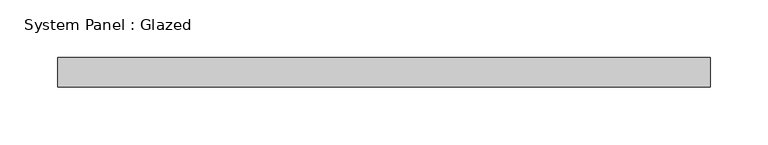
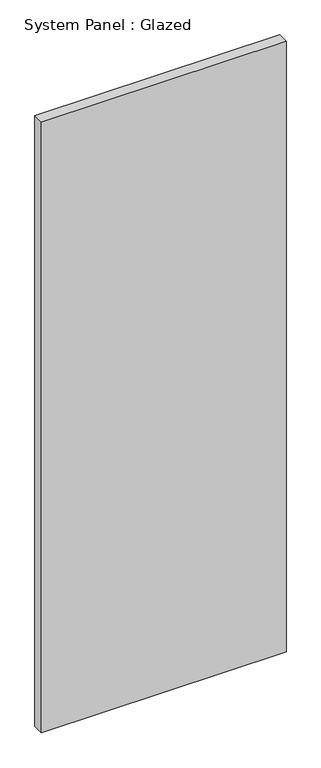
"""IFC4 building model written with IfcOpenShell, lengths in millimetres: plate geometry, System Panel : Glazed."""

from ifc_helpers import new_model, si_unit, origin, origin_with_axes, place, context, project, spatial, polyline, outline, extrude, source, transform, mapped, element, save


def system_panel_glazed_9a45502e(model_context):
    return source(origin(), model_context, "Body", "SweptSolid", [
        extrude(outline(polyline([(282.575, 19.05), (-282.575, 19.05), (-282.575, 44.45), (282.575, 44.45), (282.575, 19.05)])), origin_with_axes(), (0.0, 0.0, 1.0), 1491.023499),
    ])


if __name__ == "__main__":
    model = new_model("IFC4")
    model_context = context("Model", 3, world=origin())
    ifc_project = project(units=[si_unit("LENGTHUNIT", "METRE", prefix="MILLI")], contexts=[model_context])
    site = spatial("IfcSite", under=ifc_project)
    building = spatial("IfcBuilding", under=site)
    placement = place(None, origin())
    system_panel_glazed_shape = system_panel_glazed_9a45502e(model_context)
    element("IfcPlate", 1, ObjectType="System Panel : Glazed", at=placement, inside=building, context=model_context, shape_type="MappedRepresentation", body=[
        mapped(system_panel_glazed_shape, transform((0.0, 0.0, 0.0), x_axis=(1.0, 0.0, 0.0), y_axis=(0.0, 1.0, 0.0), z_axis=(0.0, 0.0, 1.0))),
    ])
    save(model, "model.ifc")

# Revit data of these elements
# Type "System Panel : Glazed"
#   Construction Type Id = "GSP4R"
#   Analytic Construction = "1/8 in Pilkington single glazing"
#   Visual Light Transmittance = 0.9
#   Solar Heat Gain Coefficient = 0.86
#   Heat Transfer Coefficient (U) = 1.18115 BTU/(h·ft²·°F)
#   Define Thermal Properties by = 1
# Element 1 (IfcPlate, "System Panel : Glazed")
#   Materials on its faces: "Glass"
# Materials
#   "Glass": class "Glass", colour RGB 0 128 192, transparency 0.75, Description = "Soda Lime Glass", Cost = 0
